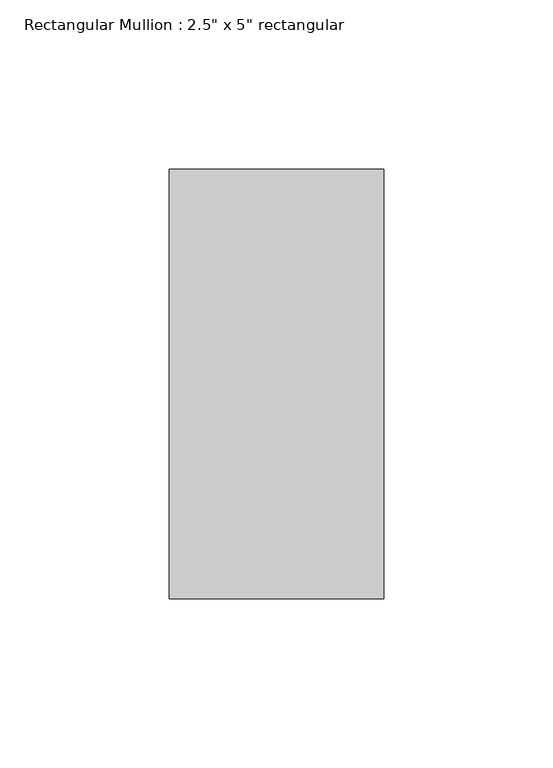
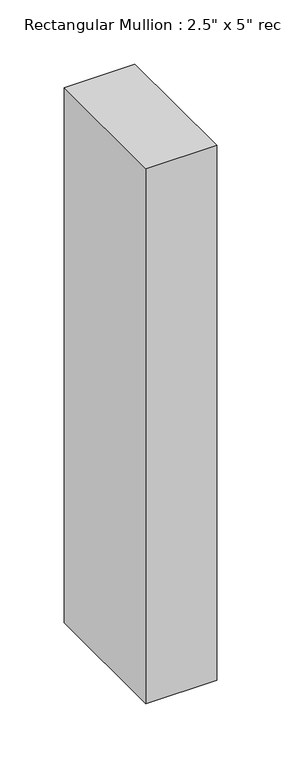
"""IFC4 building model written with IfcOpenShell, lengths in millimetres: member geometry."""

from ifc_helpers import new_model, si_unit, frame, origin, place, context, project, spatial, polyline, outline, extrude, source, transform, mapped, element, save


def member_7fd687a9(model_context):
    return source(origin(), model_context, "Body", "SweptSolid", [
        extrude(outline(polyline([(0.0, 63.5), (0.0, -63.5), (-63.5, -63.5), (-63.5, 63.5), (0.0, 63.5)])), frame((0.0, 0.0, -508.0), z_axis=(0.0, 0.0, 1.0), x_axis=(1.0, 0.0, 0.0)), (0.0, 0.0, 1.0), 508.0),
    ])


if __name__ == "__main__":
    model = new_model("IFC4")
    model_context = context("Model", 3, world=origin())
    ifc_project = project(units=[si_unit("LENGTHUNIT", "METRE", prefix="MILLI")], contexts=[model_context])
    site = spatial("IfcSite", under=ifc_project)
    building = spatial("IfcBuilding", under=site)
    placement = place(None, origin())
    member_shape = member_7fd687a9(model_context)
    element("IfcMember", 1, ObjectType="Rectangular Mullion : 2.5\" x 5\" rectangular", at=placement, inside=building, context=model_context, shape_type="MappedRepresentation", body=[
        mapped(member_shape, transform((0.0, 0.0, 0.0), x_axis=(1.0, 0.0, 0.0), y_axis=(0.0, 1.0, 0.0), z_axis=(0.0, 0.0, 1.0))),
    ])
    save(model, "model.ifc")

# Revit data of these elements
# Type "Rectangular Mullion : 2.5\" x 5\" rectangular"
#   built-in parameter 1007304 = 0.416667 (stored number, unit not read)
#   built-in parameter 1007301 = 0.104167 (stored number, unit not read)
#   built-in parameter 1007300 = 0.104167 (stored number, unit not read)
